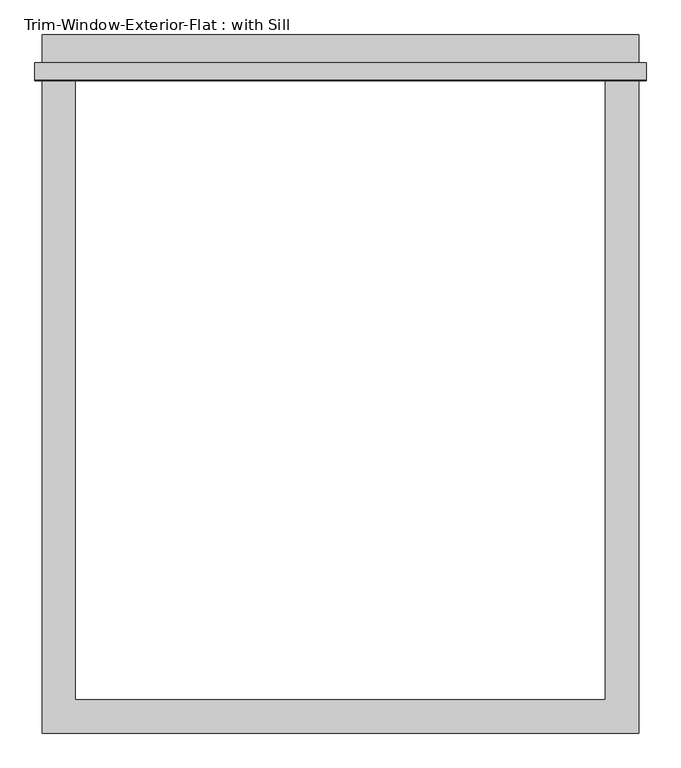
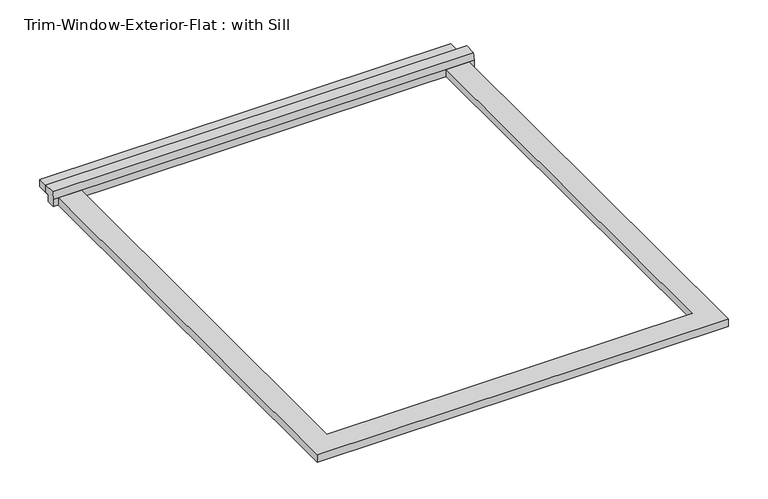
"""IFC4 building model written with IfcOpenShell, lengths in millimetres: proxy geometry, Trim-Window-Exterior-Flat : with Sill."""

from ifc_helpers import new_model, si_unit, frame, origin, origin_with_axes, place, context, project, spatial, polyline, outline, extrude, source, transform, mapped, element, save


def trim_window_exterior_flat_with_sill_0e7a59f4(model_context):
    return source(origin(), model_context, "Body", "SweptSolid", [
        extrude(outline(polyline([(514.35, 1088.9823709), (-514.35, 1088.9823709), (-514.35, 1146.1323709), (514.35, 1146.1323709), (514.35, 1088.9823709)])), origin_with_axes(), (0.0, 0.0, 1.0), 19.05),
        extrude(outline(polyline([(1098.55, 38.1), (1098.55, 19.05), (1088.9823709, 19.05), (1088.9823709, 0.0), (1066.8, 0.0), (1066.8, 19.05), (1069.2580645, 38.1), (1098.55, 38.1)])), frame((-527.05, 0.0, 0.0), z_axis=(1.0, 0.0, 0.0), x_axis=(0.0, 1.0, 0.0)), (0.0, 0.0, 1.0), 1054.1),
        extrude(outline(polyline([(-514.35, -57.15), (-514.35, 1066.8), (-457.2, 1066.8), (-457.2, 0.0), (457.2, 0.0), (457.2, 1066.8), (514.35, 1066.8), (514.35, -57.15), (-514.35, -57.15)])), origin_with_axes(), (0.0, 0.0, 1.0), 19.05),
    ])


if __name__ == "__main__":
    model = new_model("IFC4")
    model_context = context("Model", 3, world=origin())
    ifc_project = project(units=[si_unit("LENGTHUNIT", "METRE", prefix="MILLI")], contexts=[model_context])
    site = spatial("IfcSite", under=ifc_project)
    building = spatial("IfcBuilding", under=site)
    placement = place(None, origin())
    trim_window_exterior_flat_with_sill_shape = trim_window_exterior_flat_with_sill_0e7a59f4(model_context)
    element("IfcBuildingElementProxy", 1, Name="Trim-Window-Exterior-Flat : with Sill", ObjectType="Trim-Window-Exterior-Flat : with Sill", at=placement, inside=building, context=model_context, shape_type="MappedRepresentation", body=[
        mapped(trim_window_exterior_flat_with_sill_shape, transform((0.0, 0.0, 0.0), x_axis=(1.0, 0.0, 0.0), y_axis=(0.0, 1.0, 0.0), z_axis=(0.0, 0.0, 1.0))),
    ])
    save(model, "model.ifc")

# Revit data of these elements
# Type "Trim-Window-Exterior-Flat : with Sill"
#   Trim Width = 0' - 2 1/4"
#   Trim Thickness_Picture Frame = 0' - 1 1/4"
#   Trim Thickness_with Sill = 0' - 0 3/4"
#   Sill Thickness = 0' - 1 1/4"
#   Opening Width [instance default] = 2' - 0"
#   Opening Height [instance default] = 3' - 0"
#   Default Elevation = 4' - 0"
#   Sill = yes
#   Picture Frame = no
#   Trim Material [instance default] = none
# Element 1 (IfcBuildingElementProxy, "Trim-Window-Exterior-Flat : with Sill")
#   Opening Width = 3' - 0"
#   Opening Height = 3' - 6"
#   Trim Material = Clad - White
#   Materials on its faces: "Clad - White"
# Materials
#   "Clad - White": class "Wood", colour RGB 242 242 238, transparency 0, Cost = 0
